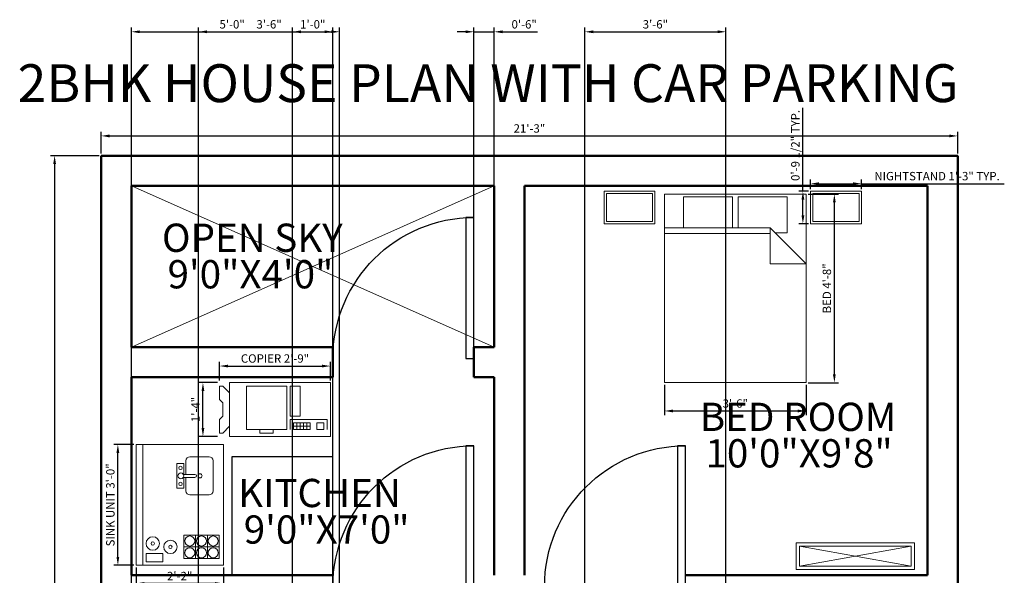
# Model space of a CAD drawing. Units: inches. Extents: x 758743 to 759108, y 3712801 to 3713581.
# Tile 4 of 4: x 758762 to 759055, y 3713415 to 3713581. Entities that reach past the tile are written whole.
import ezdxf

# ---------------------------------------------------------------- set-up
doc = ezdxf.new("R2010")
doc.units = ezdxf.units.IN
for name, color, linetype, lineweight in [('A-ANNO-DIMS', 2, 'Continuous', 18), ('A-ANNO-TEXT', 7, 'Continuous', 30), ('A-AREA-IDEN', 3, 'Continuous', 18), ('A-EQPM', 2, 'Continuous', 18), ('A-FLOR-CASE', 2, 'Continuous', 25), ('A-FLOR-FIXT', 2, 'Continuous', 18), ('A-FLOR-OPEN', 8, 'Continuous', 13), ('A-FURN', 2, 'Continuous', 18), ('DOOR', 4, 'Continuous', 25), ('WALL', 7, 'Continuous', 50)]:
    doc.layers.add(name, color=color, linetype=linetype, lineweight=lineweight)
doc.styles.get("Standard").update_dxf_attribs({"font": 'arial.ttf'})
doc.dimstyles.new('ISO-25', dxfattribs={"dimtxt": 2.5, "dimasz": 2.5, "dimexe": 1.25, "dimexo": 0.625, "dimtad": 1, "dimdec": 0, "dimlunit": 3, "dimtxsty": 'Standard', "dimcen": 2.5, "dimadec": 0, "dimazin": 0, "dimtfac": 1, "dimtdec": 0, "dimtmove": 0, "dimatfit": 3, "dimfxl": 1, "dimarcsym": 0})

# ---------------------------------------------------------------- blocks, each defined once
blk = doc.blocks.new('*U2')
for p, q in [((0, 0), (0, -100)), ((750, 0), (750, -100))]:
    blk.add_line(p, q)
blk.add_lwpolyline([(0, 0), (0, 750), (43.75, 750), (43.75, 0)], close=True)
blk.add_arc((0, 0), 750, 0, 90)
blk = doc.blocks.new('Copy Machine')
for p, q in [((0, 0), (0, -16)), ((30, 0), (0, 0)), ((30, -16), (30, 0)), ((-3, -1), (-3, -5)), ((-2, -1), (-3, -1)), ((0, -3), (-2, -1)), ((5, -1), (5, -14)), ((17, -1), (5, -1)), ((17, -14), (17, -1)), ((18, -1), (18, -10)), ((21, -1), (18, -1)), ((21, -10), (21, -1)), ((-3, -5), (-2, -6)), ((-2, -10), (-2, -6)), ((-3, -11), (-2, -10)), ((-3, -15), (-3, -11)), ((18, -10), (21, -10)), ((18, -14), (18, -11)), ((18, -11), (29, -11)), ((29, -11), (29, -14)), ((0, -13), (-2, -15)), ((5, -14), (17, -14)), ((9, -14), (9, -15)), ((13, -15), (13, -14)), ((24, -12), (19, -12)), ((19, -12), (19, -14)), ((24, -13), (19, -13)), ((19, -14), (24, -14)), ((20, -12), (20, -14)), ((21, -14), (21, -12)), ((22, -12), (22, -14)), ((23, -14), (23, -12)), ((24, -14), (24, -12)), ((28, -12), (26, -12)), ((26, -12), (26, -14)), ((26, -14), (28, -14)), ((28, -14), (28, -12)), ((-2, -15), (-3, -15)), ((0, -16), (30, -16)), ((9, -15), (13, -15))]:
    blk.add_line(p, q)
blk = doc.blocks.new('Wet Bar')
for p, q in [((0, 0), (36, 0)), ((0, -26), (0, 0)), ((36, 0), (36, -26)), ((0, -2), (36, -2)), ((3.5, -3), (1, -3)), ((1, -3), (1, -8)), ((3.5, -8), (3.5, -3)), ((1, -8), (3.5, -8)), ((2, -14.25), (9, -14.25)), ((2, -24.75), (2, -14.25)), ((5.5, -14.25), (5.5, -24.75)), ((9, -14.25), (9, -24.75)), ((26.2, -17.55), (26.2, -14.1284)), ((27.1001, -17.55), (27.1001, -14.1284)), ((2, -17.75), (9, -17.75)), ((9, -21.25), (2, -21.25)), ((36, -26), (0, -26)), ((9, -24.75), (2, -24.75))]:
    blk.add_line(p, q)
for points in [[(26.2, -14.25), (22.95, -14.25), (22.95, -12.2), (26.75, -12.2)], [(26.7487, -12.2), (30.3501, -12.2), (30.3501, -14.25), (27.1001, -14.25)], [(20.95, -21.75), (20.95, -16.05)], [(22.15, -14.85), (26.2, -14.85)], [(27.1001, -14.85), (31.15, -14.85)], [(32.3501, -16.05), (32.3501, -21.75)], [(31.15, -22.95), (22.15, -22.95)]]:
    blk.add_lwpolyline(points)
for centre, radius in [((6.5, -5), 2), ((6.5, -5), 0.5), ((5.5, -10.25), 2), ((5.5, -10.25), 0.5), ((3.75, -16), 1.5), ((7.25, -16), 1.5), ((24.25, -13.25), 0.5), ((26.65, -13.35), 0.9), ((29, -13.25), 0.5), ((3.75, -19.5), 1.5), ((7.25, -19.5), 1.5), ((26.65, -19.05), 0.6), ((3.75, -23), 1.5), ((7.25, -23), 1.5)]:
    blk.add_circle(centre, radius)
for centre, radius, start, end in [((22.2251, -16.125), 1.2772, 93.36646, 176.6335), ((26.65, -17.55), 0.45, 180, 0), ((31.075, -16.125), 1.2772, 3.366461, 86.63354), ((22.2251, -21.675), 1.2772, 183.3665, 266.6335), ((31.075, -21.675), 1.2772, 273.3665, 356.6335)]:
    blk.add_arc(centre, radius, start, end)
blk = doc.blocks.new('Bed - Queen')
for p, q in [((0, -80.00003), (0, 0)), ((0, 0), (59.99999, 0)), ((59.99999, 0), (59.99999, -80.00003)), ((7.99999, -1.2), (28.79998, -1.2)), ((7.99999, -14.4), (7.99999, -1.2)), ((28.79998, -1.2), (28.79998, -14.4)), ((31.19999, -1.2), (51.99999, -1.2)), ((31.19999, -14.4), (31.19999, -1.2)), ((51.99999, -1.2), (51.99999, -16.4)), ((0, -14.4), (44.8, -14.4)), ((59.99999, -29.6), (44.8, -14.4)), ((44.8, -14.4), (44.8, -29.6)), ((51.99999, -16.4), (46.79936, -16.4)), ((44.8, -16.8), (0, -16.8)), ((44.8, -29.6), (59.99999, -29.6)), ((59.99999, -80.00003), (0, -80.00003))]:
    blk.add_line(p, q)
blk = doc.blocks.new('*D13')
at = {"layer": 'A-ANNO-DIMS', "color": 0, "lineweight": -2, "transparency": 16777216}
for p, q in [((758785.26, 3713540.49), (758770.79, 3713540.49)), ((758772.04, 3713537.99), (758772.04, 3712841.99)), ((758785.26, 3712839.49), (758770.79, 3712839.49))]:
    blk.add_line(p, q, dxfattribs=at)
at = {"layer": 'A-ANNO-DIMS', "color": 0, "transparency": 16777216}
for points in [[(758771.62, 3713537.99), (758772.46, 3713537.99), (758772.04, 3713540.49)], [(758771.62, 3712841.99), (758772.46, 3712841.99), (758772.04, 3712839.49)]]:
    blk.add_solid(points, dxfattribs=at)
at = {"layer": 'Defpoints', "color": 0, "transparency": 16777216}
for p in [(758785.89, 3713540.49), (758772.04, 3712839.49), (758785.89, 3712839.49)]:
    blk.add_point(p, dxfattribs=at)
at = {"layer": 'A-ANNO-DIMS', "color": 0, "transparency": 16777216, "insert": (758770.14, 3713189.99), "char_height": 2.5, "attachment_point": 5, "rotation": 90}
blk.add_mtext('58\'-5"', dxfattribs=at)
blk = doc.blocks.new('*D14')
at = {"layer": 'A-ANNO-DIMS', "color": 0, "lineweight": -2, "transparency": 16777216}
for p, q in [((758785.89, 3713541.12), (758785.89, 3713547.62)), ((758788.39, 3713546.37), (759038.39, 3713546.37)), ((759040.89, 3713541.12), (759040.89, 3713547.62))]:
    blk.add_line(p, q, dxfattribs=at)
at = {"layer": 'A-ANNO-DIMS', "color": 0, "transparency": 16777216}
for points in [[(758788.39, 3713546.79), (758788.39, 3713545.95), (758785.89, 3713546.37)], [(759038.39, 3713546.79), (759038.39, 3713545.95), (759040.89, 3713546.37)]]:
    blk.add_solid(points, dxfattribs=at)
at = {"layer": 'Defpoints', "color": 0, "transparency": 16777216}
for p in [(759040.89, 3713546.37), (758785.89, 3713540.49), (759040.89, 3713540.49)]:
    blk.add_point(p, dxfattribs=at)
at = {"layer": 'A-ANNO-DIMS', "color": 0, "transparency": 16777216, "insert": (758913.39, 3713548.27), "char_height": 2.5, "attachment_point": 5}
blk.add_mtext('21\'-3"', dxfattribs=at)
blk = doc.blocks.new('NIGHTSTAND-SMALL')
for points in [[(15.15, 9.66), (15.15, 0), (0, 0), (0, 9.66)], [(14.45, 8.96), (14.45, 0.7), (0.7, 0.7), (0.7, 8.96)]]:
    blk.add_lwpolyline(points, close=True)
blk = doc.blocks.new('*D28')
at = {"layer": 'A-ANNO-DIMS', "color": 0, "lineweight": -2, "transparency": 16777216}
for p, q in [((758996.37, 3713529.06), (759005.43, 3713529.06)), ((759004.18, 3713475.37), (759004.18, 3713526.56)), ((758996.37, 3713472.87), (759005.43, 3713472.87))]:
    blk.add_line(p, q, dxfattribs=at)
at = {"layer": 'A-ANNO-DIMS', "color": 0, "transparency": 16777216}
for points in [[(759003.76, 3713526.56), (759004.59, 3713526.56), (759004.18, 3713529.06)], [(759003.76, 3713475.37), (759004.59, 3713475.37), (759004.18, 3713472.87)]]:
    blk.add_solid(points, dxfattribs=at)
at = {"layer": 'Defpoints', "color": 0, "transparency": 16777216}
for p in [(758995.75, 3713529.06), (759004.18, 3713529.06), (758995.75, 3713472.87)]:
    blk.add_point(p, dxfattribs=at)
at = {"layer": 'A-ANNO-DIMS', "color": 0, "transparency": 16777216, "insert": (759002.27, 3713500.96), "char_height": 2.5, "attachment_point": 5, "rotation": 90}
blk.add_mtext('BED 4\'-8"', dxfattribs=at)
blk = doc.blocks.new('*D29')
at = {"layer": 'A-ANNO-DIMS', "color": 0, "lineweight": -2, "transparency": 16777216}
for p, q in [((758953.61, 3713472.25), (758953.61, 3713463.2)), ((758995.75, 3713472.25), (758995.75, 3713463.2)), ((758956.11, 3713464.45), (758993.25, 3713464.45))]:
    blk.add_line(p, q, dxfattribs=at)
at = {"layer": 'A-ANNO-DIMS', "color": 0, "transparency": 16777216}
for points in [[(758956.11, 3713464.86), (758956.11, 3713464.03), (758953.61, 3713464.45)], [(758993.25, 3713464.86), (758993.25, 3713464.03), (758995.75, 3713464.45)]]:
    blk.add_solid(points, dxfattribs=at)
at = {"layer": 'Defpoints', "color": 0, "transparency": 16777216}
for p in [(758953.61, 3713472.87), (758995.75, 3713472.87), (758995.75, 3713464.45)]:
    blk.add_point(p, dxfattribs=at)
at = {"layer": 'A-ANNO-DIMS', "color": 0, "transparency": 16777216, "insert": (758974.68, 3713466.35), "char_height": 2.5, "attachment_point": 5}
blk.add_mtext('3\'-6"', dxfattribs=at)
blk = doc.blocks.new('*D32')
at = {"layer": 'A-ANNO-DIMS', "color": 0, "lineweight": -2, "transparency": 16777216}
for p, q in [((758997.08, 3713530.51), (758997.08, 3713533.4)), ((758999.58, 3713532.15), (759009.73, 3713532.15)), ((759012.23, 3713530.51), (759012.23, 3713533.4)), ((759012.23, 3713532.15), (759054.77, 3713532.15))]:
    blk.add_line(p, q, dxfattribs=at)
at = {"layer": 'A-ANNO-DIMS', "color": 0, "transparency": 16777216}
for points in [[(758999.58, 3713532.57), (758999.58, 3713531.74), (758997.08, 3713532.15)], [(759009.73, 3713532.57), (759009.73, 3713531.74), (759012.23, 3713532.15)]]:
    blk.add_solid(points, dxfattribs=at)
at = {"layer": 'Defpoints', "color": 0, "transparency": 16777216}
for p in [(759012.23, 3713532.15), (758997.08, 3713529.88), (759012.23, 3713529.88)]:
    blk.add_point(p, dxfattribs=at)
at = {"layer": 'A-ANNO-DIMS', "color": 0, "transparency": 16777216, "insert": (759034.75, 3713534.07), "char_height": 2.5, "attachment_point": 5}
blk.add_mtext('NIGHTSTAND 1\'-3" TYP.', dxfattribs=at)
blk = doc.blocks.new('*D33')
at = {"layer": 'A-ANNO-DIMS', "color": 0, "lineweight": -2, "transparency": 16777216}
for p, q in [((758994.81, 3713529.88), (758994.81, 3713554.7)), ((758996.46, 3713529.88), (758993.56, 3713529.88)), ((758994.81, 3713522.72), (758994.81, 3713527.38)), ((758996.46, 3713520.22), (758993.56, 3713520.22))]:
    blk.add_line(p, q, dxfattribs=at)
at = {"layer": 'A-ANNO-DIMS', "color": 0, "transparency": 16777216}
for points in [[(758994.39, 3713527.38), (758995.23, 3713527.38), (758994.81, 3713529.88)], [(758994.39, 3713522.72), (758995.23, 3713522.72), (758994.81, 3713520.22)]]:
    blk.add_solid(points, dxfattribs=at)
at = {"layer": 'Defpoints', "color": 0, "transparency": 16777216}
for p in [(758994.81, 3713529.88), (758997.08, 3713529.88), (758997.08, 3713520.22)]:
    blk.add_point(p, dxfattribs=at)
at = {"layer": 'A-ANNO-DIMS', "color": 0, "transparency": 16777216, "insert": (758992.89, 3713543.54), "char_height": 2.5, "attachment_point": 5, "rotation": 90}
blk.add_mtext('0\'-9 1/2" TYP.', dxfattribs=at)
blk = doc.blocks.new('*D36')
at = {"layer": 'A-ANNO-DIMS', "color": 0, "lineweight": -2, "transparency": 16777216}
for p, q in [((758821.14, 3713473.5), (758821.14, 3713479.08)), ((758854.14, 3713473.5), (758854.14, 3713479.08)), ((758823.64, 3713477.83), (758851.64, 3713477.83))]:
    blk.add_line(p, q, dxfattribs=at)
at = {"layer": 'A-ANNO-DIMS', "color": 0, "transparency": 16777216}
for points in [[(758823.64, 3713478.24), (758823.64, 3713477.41), (758821.14, 3713477.83)], [(758851.64, 3713478.24), (758851.64, 3713477.41), (758854.14, 3713477.83)]]:
    blk.add_solid(points, dxfattribs=at)
at = {"layer": 'Defpoints', "color": 0, "transparency": 16777216}
for p in [(758854.14, 3713477.83), (758821.14, 3713472.88), (758854.14, 3713472.88)]:
    blk.add_point(p, dxfattribs=at)
at = {"layer": 'A-ANNO-DIMS', "color": 0, "transparency": 16777216, "insert": (758837.64, 3713479.75), "char_height": 2.5, "attachment_point": 5}
blk.add_mtext('COPIER 2\'-9"', dxfattribs=at)
blk = doc.blocks.new('*D37')
at = {"layer": 'A-ANNO-DIMS', "color": 0, "lineweight": -2, "transparency": 16777216}
for p, q in [((758820.52, 3713472.88), (758814.94, 3713472.88)), ((758816.19, 3713459.38), (758816.19, 3713470.38)), ((758820.52, 3713456.88), (758814.94, 3713456.88))]:
    blk.add_line(p, q, dxfattribs=at)
at = {"layer": 'A-ANNO-DIMS', "color": 0, "transparency": 16777216}
for points in [[(758815.78, 3713470.38), (758816.61, 3713470.38), (758816.19, 3713472.88)], [(758815.78, 3713459.38), (758816.61, 3713459.38), (758816.19, 3713456.88)]]:
    blk.add_solid(points, dxfattribs=at)
at = {"layer": 'Defpoints', "color": 0, "transparency": 16777216}
for p in [(758816.19, 3713472.88), (758821.14, 3713472.88), (758821.14, 3713456.88)]:
    blk.add_point(p, dxfattribs=at)
at = {"layer": 'A-ANNO-DIMS', "color": 0, "transparency": 16777216, "insert": (758814.31, 3713464.88), "char_height": 2.5, "attachment_point": 5, "rotation": 90}
blk.add_mtext('1\'-4"', dxfattribs=at)
blk = doc.blocks.new('*D38')
at = {"layer": 'A-ANNO-DIMS', "color": 0, "lineweight": -2, "transparency": 16777216}
for p, q in [((758795.64, 3713454.47), (758789.62, 3713454.47)), ((758790.87, 3713420.97), (758790.87, 3713451.97)), ((758795.64, 3713418.47), (758789.62, 3713418.47))]:
    blk.add_line(p, q, dxfattribs=at)
at = {"layer": 'A-ANNO-DIMS', "color": 0, "transparency": 16777216}
for points in [[(758790.45, 3713451.97), (758791.28, 3713451.97), (758790.87, 3713454.47)], [(758790.45, 3713420.97), (758791.28, 3713420.97), (758790.87, 3713418.47)]]:
    blk.add_solid(points, dxfattribs=at)
at = {"layer": 'Defpoints', "color": 0, "transparency": 16777216}
for p in [(758790.87, 3713454.47), (758796.27, 3713454.47), (758796.27, 3713418.47)]:
    blk.add_point(p, dxfattribs=at)
at = {"layer": 'A-ANNO-DIMS', "color": 0, "transparency": 16777216, "insert": (758788.95, 3713436.47), "char_height": 2.5, "attachment_point": 5, "rotation": 90}
blk.add_mtext('SINK UNIT 3\'-0"', dxfattribs=at)
blk = doc.blocks.new('*D39')
at = {"layer": 'A-ANNO-DIMS', "color": 0, "lineweight": -2, "transparency": 16777216}
for p, q in [((758796.27, 3713417.84), (758796.27, 3713411.82)), ((758822.27, 3713417.84), (758822.27, 3713411.82)), ((758819.77, 3713413.07), (758798.77, 3713413.07))]:
    blk.add_line(p, q, dxfattribs=at)
at = {"layer": 'A-ANNO-DIMS', "color": 0, "transparency": 16777216}
for points in [[(758798.77, 3713413.48), (758798.77, 3713412.65), (758796.27, 3713413.07)], [(758819.77, 3713413.48), (758819.77, 3713412.65), (758822.27, 3713413.07)]]:
    blk.add_solid(points, dxfattribs=at)
at = {"layer": 'Defpoints', "color": 0, "transparency": 16777216}
for p in [(758796.27, 3713418.47), (758822.27, 3713418.47), (758796.27, 3713413.07)]:
    blk.add_point(p, dxfattribs=at)
at = {"layer": 'A-ANNO-DIMS', "color": 0, "transparency": 16777216, "insert": (758809.27, 3713414.95), "char_height": 2.5, "attachment_point": 5}
blk.add_mtext('2\'-2"', dxfattribs=at)
blk = doc.blocks.new('*D46')
at = {"layer": 'A-ANNO-DIMS', "color": 0, "lineweight": -2, "transparency": 16777216}
for p, q in [((758842.89, 3712849.12), (758842.89, 3713578.64)), ((758854.89, 3712849.12), (758854.89, 3713578.64)), ((758845.39, 3713577.39), (758852.39, 3713577.39))]:
    blk.add_line(p, q, dxfattribs=at)
at = {"layer": 'A-ANNO-DIMS', "color": 0, "transparency": 16777216}
for points in [[(758845.39, 3713577.81), (758845.39, 3713576.97), (758842.89, 3713577.39)], [(758852.39, 3713577.81), (758852.39, 3713576.97), (758854.89, 3713577.39)]]:
    blk.add_solid(points, dxfattribs=at)
at = {"layer": 'Defpoints', "color": 0, "transparency": 16777216}
for p in [(758854.89, 3713577.39), (758842.89, 3712848.49), (758854.89, 3712848.49)]:
    blk.add_point(p, dxfattribs=at)
at = {"layer": 'A-ANNO-DIMS', "color": 0, "transparency": 16777216, "insert": (758848.89, 3713579.29), "char_height": 2.5, "attachment_point": 5}
blk.add_mtext('1\'-0"', dxfattribs=at)
blk = doc.blocks.new('*D49')
at = {"layer": 'A-ANNO-DIMS', "color": 0, "lineweight": -2, "transparency": 16777216}
for p, q in [((758929.89, 3713089.12), (758929.89, 3713578.64)), ((758971.89, 3713089.12), (758971.89, 3713578.64)), ((758932.39, 3713577.39), (758969.39, 3713577.39))]:
    blk.add_line(p, q, dxfattribs=at)
at = {"layer": 'A-ANNO-DIMS', "color": 0, "transparency": 16777216}
for points in [[(758932.39, 3713577.81), (758932.39, 3713576.97), (758929.89, 3713577.39)], [(758969.39, 3713577.81), (758969.39, 3713576.97), (758971.89, 3713577.39)]]:
    blk.add_solid(points, dxfattribs=at)
at = {"layer": 'Defpoints', "color": 0, "transparency": 16777216}
for p in [(758971.89, 3713577.39), (758929.89, 3713088.49), (758971.89, 3713088.49)]:
    blk.add_point(p, dxfattribs=at)
at = {"layer": 'A-ANNO-DIMS', "color": 0, "transparency": 16777216, "insert": (758950.89, 3713579.29), "char_height": 2.5, "attachment_point": 5}
blk.add_mtext('3\'-6"', dxfattribs=at)
blk = doc.blocks.new('*D51')
at = {"layer": 'A-ANNO-DIMS', "color": 0, "lineweight": -2, "transparency": 16777216}
for p, q in [((758814.89, 3713314.12), (758814.89, 3713578.64)), ((758856.89, 3713314.12), (758856.89, 3713578.64)), ((758817.39, 3713577.39), (758854.39, 3713577.39))]:
    blk.add_line(p, q, dxfattribs=at)
at = {"layer": 'A-ANNO-DIMS', "color": 0, "transparency": 16777216}
for points in [[(758817.39, 3713577.81), (758817.39, 3713576.97), (758814.89, 3713577.39)], [(758854.39, 3713577.81), (758854.39, 3713576.97), (758856.89, 3713577.39)]]:
    blk.add_solid(points, dxfattribs=at)
at = {"layer": 'Defpoints', "color": 0, "transparency": 16777216}
for p in [(758856.89, 3713577.39), (758814.89, 3713313.49), (758856.89, 3713313.49)]:
    blk.add_point(p, dxfattribs=at)
at = {"layer": 'A-ANNO-DIMS', "color": 0, "transparency": 16777216, "insert": (758835.89, 3713579.29), "char_height": 2.5, "attachment_point": 5}
blk.add_mtext('3\'-6"', dxfattribs=at)
blk = doc.blocks.new('*D53')
at = {"layer": 'A-ANNO-DIMS', "color": 0, "lineweight": -2, "transparency": 16777216}
for p, q in [((758794.89, 3713407.12), (758794.89, 3713578.64)), ((758854.89, 3713407.12), (758854.89, 3713578.64)), ((758797.39, 3713577.39), (758852.39, 3713577.39))]:
    blk.add_line(p, q, dxfattribs=at)
at = {"layer": 'A-ANNO-DIMS', "color": 0, "transparency": 16777216}
for points in [[(758797.39, 3713577.81), (758797.39, 3713576.97), (758794.89, 3713577.39)], [(758852.39, 3713577.81), (758852.39, 3713576.97), (758854.89, 3713577.39)]]:
    blk.add_solid(points, dxfattribs=at)
at = {"layer": 'Defpoints', "color": 0, "transparency": 16777216}
for p in [(758854.89, 3713577.39), (758794.89, 3713406.49), (758854.89, 3713406.49)]:
    blk.add_point(p, dxfattribs=at)
at = {"layer": 'A-ANNO-DIMS', "color": 0, "transparency": 16777216, "insert": (758824.89, 3713579.29), "char_height": 2.5, "attachment_point": 5}
blk.add_mtext('5\'-0"', dxfattribs=at)
blk = doc.blocks.new('*D60')
at = {"layer": 'A-ANNO-DIMS', "color": 0, "lineweight": -2, "transparency": 16777216}
for p, q in [((758896.89, 3713484.12), (758896.89, 3713578.64)), ((758902.89, 3713484.12), (758902.89, 3713578.64)), ((758894.39, 3713577.39), (758891.89, 3713577.39)), ((758896.89, 3713577.39), (758902.89, 3713577.39)), ((758905.39, 3713577.39), (758915.78, 3713577.39))]:
    blk.add_line(p, q, dxfattribs=at)
at = {"layer": 'A-ANNO-DIMS', "color": 0, "transparency": 16777216}
for points in [[(758894.39, 3713577.81), (758894.39, 3713576.97), (758896.89, 3713577.39)], [(758905.39, 3713577.81), (758905.39, 3713576.97), (758902.89, 3713577.39)]]:
    blk.add_solid(points, dxfattribs=at)
at = {"layer": 'Defpoints', "color": 0, "transparency": 16777216}
for p in [(758902.89, 3713577.39), (758896.89, 3713483.49), (758902.89, 3713483.49)]:
    blk.add_point(p, dxfattribs=at)
at = {"layer": 'A-ANNO-DIMS', "color": 0, "transparency": 16777216, "insert": (758911.83, 3713579.29), "char_height": 2.5, "attachment_point": 5}
blk.add_mtext('0\'-6"', dxfattribs=at)

msp = doc.modelspace()

# ---------------------------------------------------------------- linework, layer by layer
at = {"layer": 'A-FLOR-CASE'}
for p, q in [((758854.89, 3713450.84), (758854.89, 3713473.68)), ((758824.89, 3713415.49), (758824.89, 3713450.84)), ((758824.89, 3713450.84), (758854.89, 3713450.84))]:
    msp.add_line(p, q, dxfattribs=at)
at = {"layer": 'A-FLOR-OPEN'}
for p, q in [((758794.89, 3713531.49), (758902.89, 3713483.49)), ((758794.89, 3713483.49), (758902.89, 3713531.49))]:
    msp.add_line(p, q, dxfattribs=at)
at = {"layer": 'A-FURN'}
for p, q in [((758993.76, 3713418.22), (759027.02, 3713424.16)), ((759027.02, 3713418.22), (758993.76, 3713424.16))]:
    msp.add_line(p, q, dxfattribs=at)
for points in [[(758992.76, 3713417.22), (759028.02, 3713417.22), (759028.02, 3713425.16), (758992.76, 3713425.16)], [(758993.76, 3713418.22), (759027.02, 3713418.22), (759027.02, 3713424.16), (758993.76, 3713424.16)]]:
    msp.add_lwpolyline(points, close=True, dxfattribs=at)
at = {"layer": 'WALL'}
for p, q in [((758785.89, 3713540.49), (759040.89, 3713540.49)), ((758785.89, 3713540.49), (758785.89, 3712839.49)), ((759040.89, 3713540.49), (759040.89, 3712839.49)), ((758794.89, 3713531.49), (758794.89, 3713483.49)), ((758794.89, 3713531.49), (758902.89, 3713531.49)), ((758902.89, 3713531.49), (758902.89, 3713483.49)), ((758911.89, 3713531.49), (758911.89, 3713415.49)), ((758911.89, 3713531.49), (759031.89, 3713531.49)), ((759031.89, 3713531.49), (759031.89, 3713415.49)), ((758794.89, 3713483.49), (758854.89, 3713483.49)), ((758854.89, 3713483.49), (758854.89, 3713474.49)), ((758896.89, 3713483.49), (758896.89, 3713474.49)), ((758896.89, 3713483.49), (758902.89, 3713483.49)), ((758794.89, 3713474.49), (758854.89, 3713474.49)), ((758794.89, 3713474.49), (758794.89, 3713415.49)), ((758896.89, 3713474.49), (758902.89, 3713474.49)), ((758902.89, 3713474.49), (758902.89, 3713415.49)), ((758794.89, 3713415.49), (758854.89, 3713415.49)), ((758959.89, 3713415.49), (759031.89, 3713415.49))]:
    msp.add_line(p, q, dxfattribs=at)

# ---------------------------------------------------------------- block references
at = {"layer": 'A-EQPM'}
msp.add_blockref('Copy Machine', (758824.14, 3713472.88), dxfattribs=at)
at = {"layer": 'A-FLOR-FIXT', "rotation": 90}
msp.add_blockref('Wet Bar', (758796.27, 3713418.47), dxfattribs=at)
at = {"layer": 'A-FURN'}
for p in [(758935.61, 3713520.22), (758997.08, 3713520.22)]:
    msp.add_blockref('NIGHTSTAND-SMALL', p, dxfattribs=at)
at = {"layer": 'A-FURN', "xscale": 0.7022725675296493, "yscale": 0.7022725675296493, "zscale": 0.7022725675296493}
msp.add_blockref('Bed - Queen', (758953.61, 3713529.06), dxfattribs=at)
at = {"layer": 'DOOR', "xscale": -0.0559999999999739, "yscale": 0.0559999999999739, "zscale": 0.0559999999999739}
for p in [(758896.89, 3713480.09), (758896.89, 3713412.09), (758959.89, 3713412.09)]:
    msp.add_blockref('*U2', p, dxfattribs=at)

# ---------------------------------------------------------------- texts
at = {"layer": 'A-ANNO-TEXT'}
msp.add_text('2BHK HOUSE PLAN WITH CAR PARKING', height=11.2839, dxfattribs=at).set_placement((758761.02, 3713556.44))
at = {"layer": 'A-AREA-IDEN'}
for s, p in [('OPEN SKY', (758803.99, 3713511.83)), ('9\'0"X4\'0"', (758805.66, 3713500.96)), ('BED ROOM', (758964.13, 3713458.49)), ('10\'0"X9\'8"', (758965.8, 3713447.62)), ('KITCHEN', (758826.67, 3713435.8)), ('9\'0"X7\'0"', (758828.34, 3713424.92))]:
    msp.add_text(s, height=8.421, dxfattribs=at).set_placement(p)

# ---------------------------------------------------------------- dimensions: what is measured, and where the dimension line sits
at = {"layer": 'A-ANNO-DIMS'}
for base, p1, p2, override, picture, middle in [((758854.89, 3713577.39), (758794.89, 3713406.49), (758854.89, 3713406.49), {"dimdec": 1, "dimlfac": 1, "dimrnd": 0, "dimzin": 1, "dimdsep": 46, "dimlunit": 4, "dimfrac": 2}, '*D53', (758824.89, 3713579.29)), ((758856.89, 3713577.39), (758814.89, 3713313.49), (758856.89, 3713313.49), {"dimdec": 1, "dimlfac": 1, "dimrnd": 0, "dimzin": 1, "dimdsep": 46, "dimlunit": 4, "dimfrac": 2}, '*D51', (758835.89, 3713579.29)), ((758854.89, 3713577.39), (758842.89, 3712848.49), (758854.89, 3712848.49), {"dimdec": 1, "dimlfac": 1, "dimrnd": 0, "dimzin": 1, "dimdsep": 46, "dimlunit": 4, "dimfrac": 2}, '*D46', (758848.89, 3713579.29)), ((758902.89, 3713577.39), (758896.89, 3713483.49), (758902.89, 3713483.49), {"dimdec": 1, "dimlfac": 1, "dimrnd": 0, "dimzin": 1, "dimdsep": 46, "dimlunit": 4, "dimfrac": 2}, '*D60', (758911.83, 3713579.29)), ((758971.89, 3713577.39), (758929.89, 3713088.49), (758971.89, 3713088.49), {"dimdec": 1, "dimlfac": 1, "dimrnd": 0, "dimzin": 1, "dimdsep": 46, "dimlunit": 4, "dimfrac": 2}, '*D49', (758950.89, 3713579.29)), ((759040.89, 3713546.37), (758785.89, 3713540.49), (759040.89, 3713540.49), {"dimclrd": 0, "dimclre": 0, "dimclrt": 0}, '*D14', (758913.39, 3713548.27)), ((758995.75, 3713464.45), (758953.61, 3713472.87), (758995.75, 3713472.87), {"dimdec": 1, "dimlfac": 1, "dimrnd": 0, "dimzin": 1, "dimdsep": 46, "dimlunit": 4, "dimfrac": 2}, '*D29', (758974.68, 3713466.35))]:
    dim = msp.add_linear_dim(base=base, p1=p1, p2=p2, dimstyle='ISO-25', override=override, dxfattribs=at)
    dim.commit()
    dim.dimension.update_dxf_attribs({"geometry": picture, "text_midpoint": middle})
for base, p1, p2, text, picture, middle in [((758994.81, 3713529.88), (758997.08, 3713520.22), (758997.08, 3713529.88), '<> TYP.', '*D33', (758992.89, 3713543.54)), ((759004.18, 3713529.06), (758995.75, 3713472.87), (758995.75, 3713529.06), 'BED <>', '*D28', (759002.27, 3713500.96)), ((758790.87, 3713454.47), (758796.27, 3713418.47), (758796.27, 3713454.47), 'SINK UNIT <>', '*D38', (758788.95, 3713436.47))]:
    dim = msp.add_linear_dim(base=base, p1=p1, p2=p2, angle=90, text=text, dimstyle='ISO-25', override={"dimdec": 1, "dimlfac": 1, "dimrnd": 0, "dimzin": 1, "dimdsep": 46, "dimlunit": 4, "dimfrac": 2}, dxfattribs=at)
    dim.commit()
    dim.dimension.update_dxf_attribs({"geometry": picture, "text_midpoint": middle})
for base, p1, p2, angle, override, picture, middle in [((758772.04, 3712839.49), (758785.89, 3713540.49), (758785.89, 3712839.49), 90, {"dimclrd": 0, "dimclre": 0, "dimclrt": 0}, '*D13', (758770.14, 3713189.99)), ((758816.19, 3713472.88), (758821.14, 3713456.88), (758821.14, 3713472.88), 90, {"dimdec": 1, "dimlfac": 1, "dimrnd": 0, "dimzin": 1, "dimdsep": 46, "dimlunit": 4, "dimfrac": 2}, '*D37', (758814.31, 3713464.88)), ((758796.27, 3713413.07), (758822.27, 3713418.47), (758796.27, 3713418.47), 180, {"dimdec": 1, "dimlfac": 1, "dimrnd": 0, "dimzin": 1, "dimdsep": 46, "dimlunit": 4, "dimfrac": 2}, '*D39', (758809.27, 3713414.95))]:
    dim = msp.add_linear_dim(base=base, p1=p1, p2=p2, angle=angle, dimstyle='ISO-25', override=override, dxfattribs=at)
    dim.commit()
    dim.dimension.update_dxf_attribs({"geometry": picture, "text_midpoint": middle})
for base, p1, p2, text, picture, middle in [((759012.2316, 3713532.1532), (758997.0836, 3713529.881), (759012.2316, 3713529.881), 'NIGHTSTAND <> TYP.', '*D32', (759034.7512, 3713534.0717)), ((758854.14, 3713477.83), (758821.14, 3713472.88), (758854.14, 3713472.88), 'COPIER <>', '*D36', (758837.64, 3713479.75))]:
    dim = msp.add_linear_dim(base=base, p1=p1, p2=p2, text=text, dimstyle='ISO-25', override={"dimdec": 1, "dimlfac": 1, "dimrnd": 0, "dimzin": 1, "dimdsep": 46, "dimlunit": 4, "dimfrac": 2}, dxfattribs=at)
    dim.commit()
    dim.dimension.update_dxf_attribs({"geometry": picture, "text_midpoint": middle})

doc.saveas('drawing.dxf')
